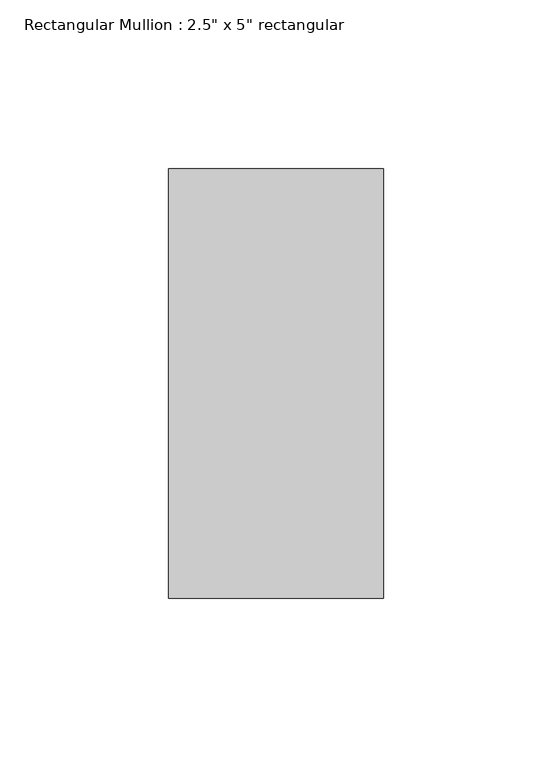
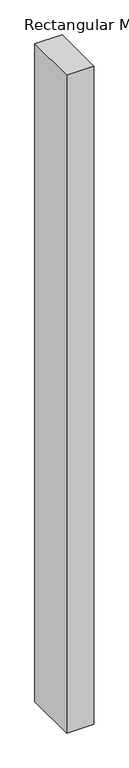
"""IFC4 building model written with IfcOpenShell, lengths in millimetres: member geometry."""

from ifc_helpers import new_model, si_unit, frame, origin, place, context, project, spatial, polyline, outline, extrude, source, transform, mapped, element, save


def member_8cf20c82(model_context):
    return source(origin(), model_context, "Body", "SweptSolid", [
        extrude(outline(polyline([(0.0, 63.5), (0.0, -63.5), (-63.5, -63.5), (-63.5, 63.5), (0.0, 63.5)])), frame((0.0, 0.0, -1610.0660092), z_axis=(0.0, 0.0, 1.0), x_axis=(1.0, 0.0, 0.0)), (0.0, 0.0, 1.0), 1610.0660092),
    ])


if __name__ == "__main__":
    model = new_model("IFC4")
    model_context = context("Model", 3, world=origin())
    ifc_project = project(units=[si_unit("LENGTHUNIT", "METRE", prefix="MILLI")], contexts=[model_context])
    site = spatial("IfcSite", under=ifc_project)
    building = spatial("IfcBuilding", under=site)
    placement = place(None, origin())
    member_shape = member_8cf20c82(model_context)
    element("IfcMember", 1, ObjectType="Rectangular Mullion : 2.5\" x 5\" rectangular", at=placement, inside=building, context=model_context, shape_type="MappedRepresentation", body=[
        mapped(member_shape, transform((0.0, 0.0, 0.0), x_axis=(1.0, 0.0, 0.0), y_axis=(0.0, 1.0, 0.0), z_axis=(0.0, 0.0, 1.0))),
    ])
    save(model, "model.ifc")

# Revit data of these elements
# Type "Rectangular Mullion : 2.5\" x 5\" rectangular"
#   built-in parameter 1007304 = 0.416667 (stored number, unit not read)
#   built-in parameter 1007301 = 0.104167 (stored number, unit not read)
#   built-in parameter 1007300 = 0.104167 (stored number, unit not read)
# Element 1 (IfcMember, "Rectangular Mullion : 2.5\" x 5\" rectangular")
#   Materials on its faces: "Aluminum"
# Materials
#   "Aluminum": class "Metal", colour RGB 247 247 247, transparency 0, Description = "Aluminum 6061", Cost = 0
